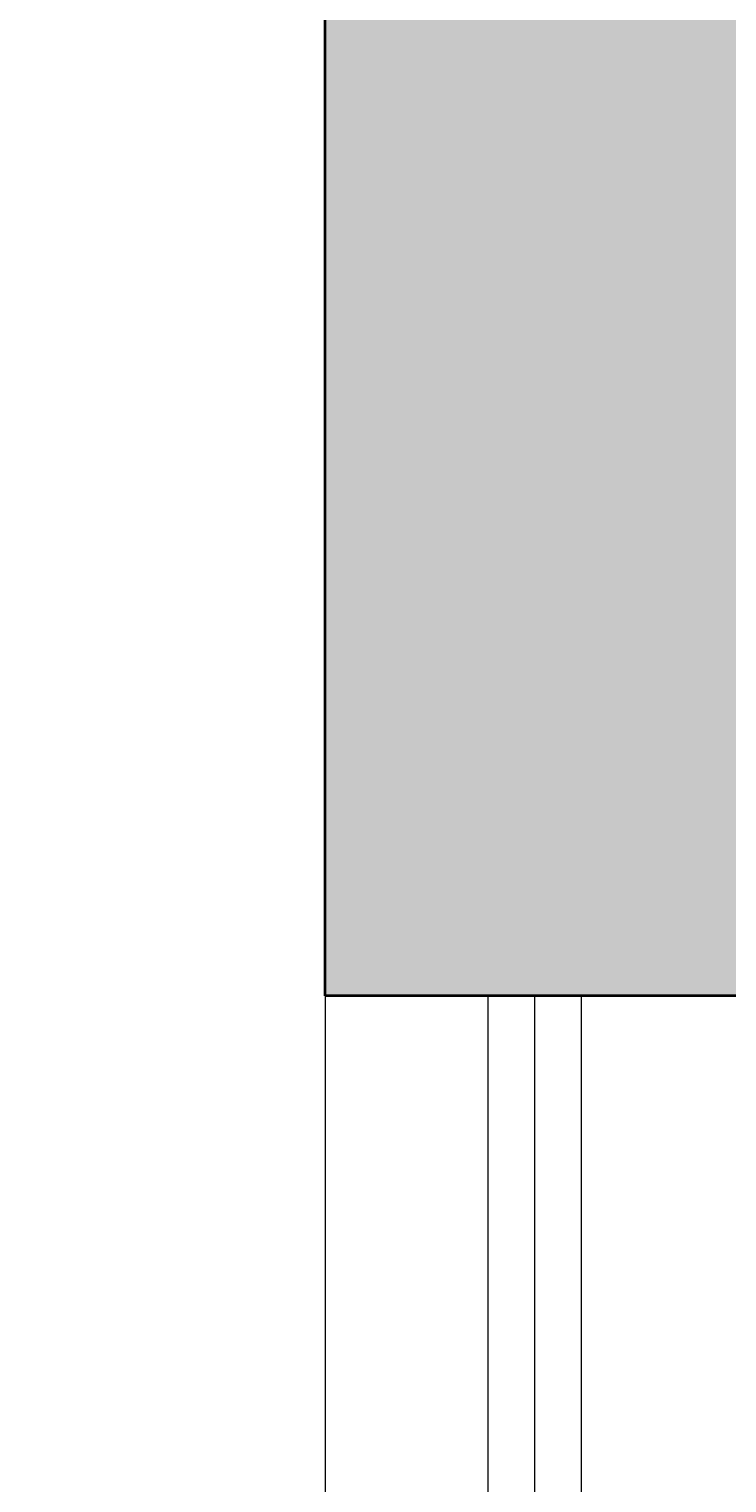
# Model space of a CAD drawing. Units: inches. Extents: x 84 to 1044, y -280 to 906.
# Tile 74 of 105: x 689 to 704, y 481 to 512. Entities that reach past the tile are written whole.
import ezdxf

# ---------------------------------------------------------------- set-up
doc = ezdxf.new("R2010")
doc.units = ezdxf.units.IN
for name, color, linetype, lineweight in [('A-ANNO-DIMS', 2, 'Continuous', 18), ('WALL', 250, 'Continuous', 35), ('WINDOW', 160, 'Continuous', 13)]:
    doc.layers.add(name, color=color, linetype=linetype, lineweight=lineweight)
doc.layers.add('A-WALL-PATT', color=251, linetype='Continuous', lineweight=9, true_color=0x636466)
doc.styles.get("Standard").update_dxf_attribs({"font": 'arial.ttf'})
doc.dimstyles.get("Standard").update_dxf_attribs({"dimtxt": 0.18, "dimasz": 0.18, "dimexe": 0.18, "dimexo": 0.0625, "dimgap": 0.09, "dimtad": 0, "dimtih": 1, "dimtoh": 1, "dimdec": 4, "dimzin": 0, "dimdsep": 46, "dimtxsty": 'Standard', "dimcen": 0.09, "dimadec": 0, "dimazin": 0, "dimtfac": 1, "dimtdec": 4, "dimtofl": 0, "dimtmove": 0, "dimatfit": 3, "dimfxl": 1, "dimtolj": 1, "dimtzin": 0, "dimarcsym": 0})

# ---------------------------------------------------------------- blocks, each defined once
blk = doc.blocks.new('WIN-72IN')
for p, q in [((72.004, 5.5), (0.004, 5.5)), ((72.004, 4.5), (0.004, 4.5)), ((72.004, 3.5), (0.004, 3.5)), ((0.004, 0), (72.004, 0))]:
    blk.add_line(p, q)
blk = doc.blocks.new('*D62')
at = {"layer": 'A-ANNO-DIMS', "color": 0, "lineweight": -2, "transparency": 16777216}
for p, q in [((203.179, 709.183), (203.179, 905.9)), ((896.074, 400.183), (896.074, 905.9)), ((203.359, 905.72), (549.232, 905.72)), ((895.894, 905.72), (550.021, 905.72))]:
    blk.add_line(p, q, dxfattribs=at)
at = {"layer": 'A-ANNO-DIMS', "color": 0, "transparency": 16777216}
for points in [[(203.359, 905.75), (203.359, 905.69), (203.179, 905.72)], [(895.894, 905.75), (895.894, 905.69), (896.074, 905.72)]]:
    blk.add_solid(points, dxfattribs=at)
at = {"layer": 'Defpoints', "color": 0, "transparency": 16777216}
for p in [(896.074, 905.72), (203.179, 709.12), (896.074, 400.12)]:
    blk.add_point(p, dxfattribs=at)
at = {"layer": 'A-ANNO-DIMS', "color": 0, "transparency": 16777216, "insert": (549.627, 905.72), "char_height": 0.18, "attachment_point": 5}
blk.add_mtext('\\A1;692.9', dxfattribs=at)

msp = doc.modelspace()

# ---------------------------------------------------------------- hatches: boundary and pattern name
at = {"layer": 'A-WALL-PATT', "transparency": 33554597}
h = msp.add_hatch(color=256, dxfattribs=at)
h.dxf.hatch_style = 1
h.paths.add_polyline_path([(671.074, 100.12), (647.074, 100.12), (647.074, 160.12), (641.074, 160.12), (620.824, 160.12), (620.824, 151.12), (638.074, 151.12), (638.074, 91.12), (671.074, 91.12)])
h.paths.add_polyline_path([(791.074, 100.12), (743.074, 100.12), (743.074, 91.12), (791.074, 91.12)])
h.paths.add_polyline_path([(896.074, 346.12), (887.074, 346.12), (887.074, 334.12), (870.955, 334.12), (833.074, 334.12), (804.574, 334.12), (804.574, 328.12), (887.074, 328.12), (887.074, 100.12), (863.074, 100.12), (863.074, 91.12), (896.074, 91.12)])
h.paths.add_polyline_path([(507.574, 154.729), (507.574, 160.12), (464.074, 160.12), (464.074, 247.12), (641.074, 247.12), (641.074, 208.12), (647.074, 208.12), (647.074, 328.12), (659.074, 328.12), (659.074, 334.12), (617.074, 334.12), (617.074, 328.12), (641.074, 328.12), (641.074, 256.12), (545.074, 256.12), (545.074, 328.12), (569.074, 328.12), (569.074, 334.12), (518.074, 334.12), (518.074, 325.12), (536.074, 325.12), (536.074, 256.12), (464.074, 256.12), (464.074, 325.12), (482.074, 325.12), (482.074, 334.12), (455.074, 334.12), (455.074, 160.12), (413.127, 160.12), (413.127, 151.12), (455.074, 151.12), (455.074, 91.12), (464.074, 91.12), (464.074, 151.12), (507.574, 151.12)])
h.paths.add_polyline_path([(572.824, 160.12), (555.574, 160.12), (555.574, 151.12), (572.824, 151.12)], flags=17)
h.paths.add_polyline_path([(341.127, 160.12), (299.179, 160.12), (299.179, 211.12), (294.179, 211.12), (290.179, 211.12), (290.179, 151.12), (341.127, 151.12)])
h.paths.add_polyline_path([(299.179, 256.12), (212.179, 256.12), (212.179, 274.12), (203.179, 274.12), (203.179, 247.12), (299.179, 247.12)])
h.paths.add_polyline_path([(212.179, 514.12), (398.074, 514.12), (398.074, 519.12), (398.074, 520.12), (212.179, 520.12), (212.179, 574.12), (203.179, 574.12), (203.179, 310.12), (212.179, 310.12), (212.179, 328.12), (290.179, 328.12), (290.179, 292.12), (299.179, 292.12), (299.179, 328.12), (332.179, 328.12), (332.179, 334.12), (212.179, 334.12)])
h.paths.add_polyline_path([(287.127, 709.12), (203.179, 709.12), (203.179, 646.12), (212.179, 646.12), (212.179, 700.12), (287.127, 700.12)])
h.paths.add_polyline_path([(470.074, 709.12), (359.127, 709.12), (359.127, 700.12), (434.074, 700.12), (434.074, 574.12), (440.074, 574.12), (440.074, 622.12), (464.074, 622.12), (464.074, 628.12), (440.074, 628.12), (440.074, 700.12), (470.074, 700.12)])
h.paths.add_polyline_path([(572.074, 709.12), (506.074, 709.12), (506.074, 700.12), (536.074, 700.12), (536.074, 628.12), (494.074, 628.12), (494.074, 622.12), (536.074, 622.12), (536.074, 520.12), (440.074, 520.12), (440.074, 544.12), (434.074, 544.12), (434.074, 514.12), (644.074, 514.12), (644.074, 519.12), (644.074, 544.12), (638.074, 544.12), (638.074, 520.12), (542.074, 520.12), (542.074, 622.12), (584.074, 622.12), (584.074, 628.12), (542.074, 628.12), (542.074, 700.12), (572.074, 700.12)])
h.paths.add_polyline_path([(698.074, 709.12), (608.074, 709.12), (608.074, 700.12), (638.074, 700.12), (638.074, 628.12), (614.074, 628.12), (614.074, 622.12), (638.074, 622.12), (638.074, 574.12), (644.074, 574.12), (644.074, 700.12), (698.074, 700.12)])
h.paths.add_polyline_path([(833.074, 709.12), (770.074, 709.12), (770.074, 700.12), (824.074, 700.12), (824.074, 646.12), (833.074, 646.12)])
h.paths.add_polyline_path([(833.074, 574.12), (824.074, 574.12), (824.074, 520.12), (791.244, 520.12), (712.904, 520.12), (680.074, 520.12), (680.074, 514.12), (695.074, 514.12), (695.074, 491.62), (704.074, 491.62), (704.074, 511.12), (833.074, 511.12)])
h.paths.add_polyline_path([(704.074, 419.62), (695.074, 419.62), (695.074, 370.12), (704.074, 370.12)])
h.paths.add_polyline_path([(896.074, 400.12), (833.074, 400.12), (833.074, 364.12), (839.074, 364.12), (839.074, 394.12), (887.074, 394.12), (887.074, 382.12), (896.074, 382.12)])
h.paths.add_polyline_path([(732.574, 334.12), (695.074, 334.12), (695.074, 328.12), (732.574, 328.12)])

# ---------------------------------------------------------------- linework, layer by layer
at = {"layer": 'WALL'}
for p, q in [((695.074, 491.62), (695.074, 514.12)), ((704.074, 491.62), (695.074, 491.62))]:
    msp.add_line(p, q, dxfattribs=at)

# ---------------------------------------------------------------- block references
at = {"layer": 'WINDOW', "rotation": 270.0000000000001}
msp.add_blockref('WIN-72IN', (695.074, 491.624), dxfattribs=at)

# ---------------------------------------------------------------- dimensions: what is measured, and where the dimension line sits
at = {"layer": 'A-ANNO-DIMS'}
dim = msp.add_linear_dim(base=(896.074, 905.72), p1=(203.179, 709.12), p2=(896.074, 400.12), dimstyle='Standard', override={"dimdec": 1, "dimlfac": 1, "dimrnd": 0, "dimzin": 0, "dimdsep": 46, "dimlunit": 2}, dxfattribs=at)
dim.commit()
dim.dimension.update_dxf_attribs({"geometry": '*D62', "text_midpoint": (549.627, 905.72)})

doc.saveas('drawing.dxf')
